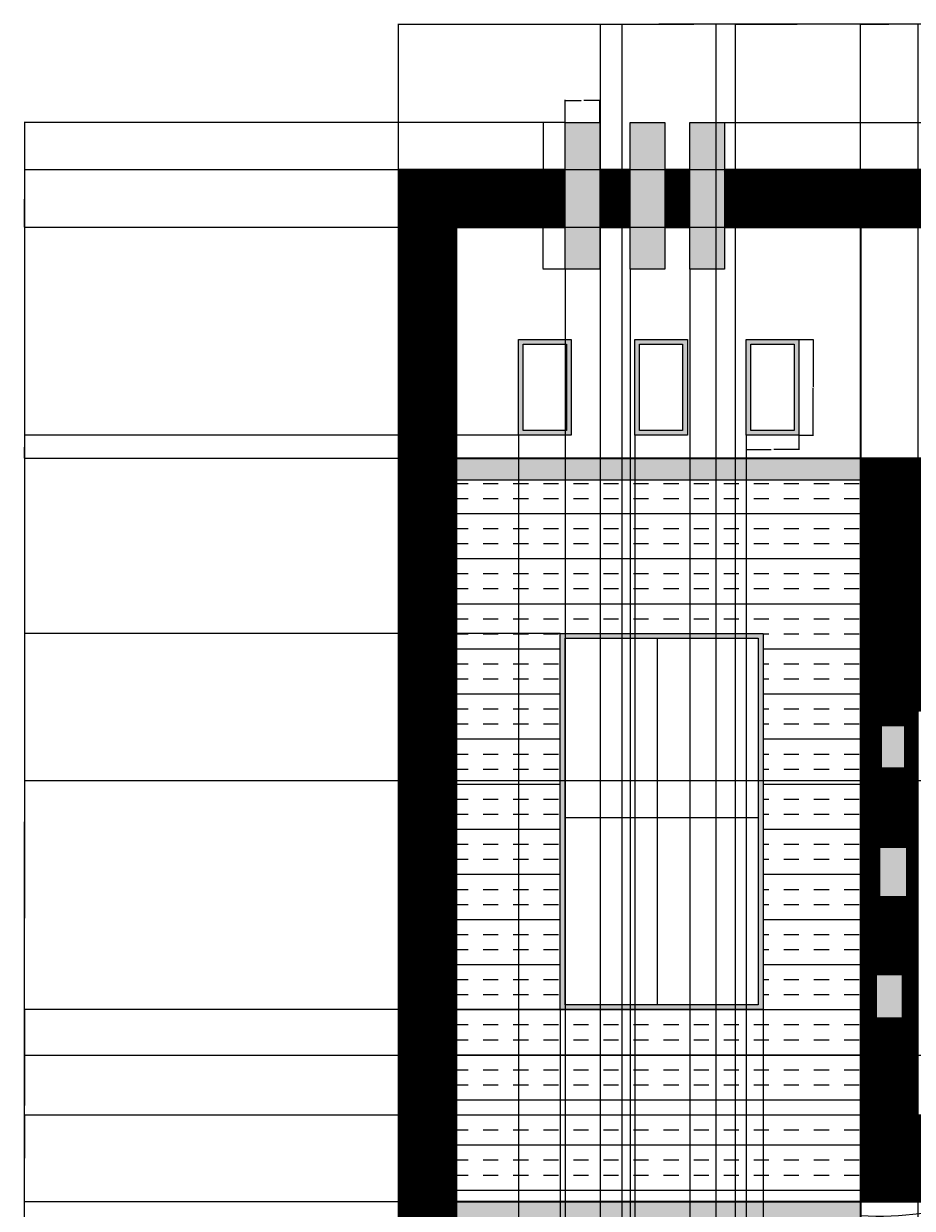
# Model space of a CAD drawing. Units: inches. Extents: x 484 to 1264, y 95 to 991.
# Tile 7 of 8: x 484 to 853, y 499 to 991. Entities that reach past the tile are written whole.
import ezdxf

# ---------------------------------------------------------------- set-up
doc = ezdxf.new("R2010")
doc.units = ezdxf.units.IN
doc.header["$MEASUREMENT"] = 0
for name, color, linetype, lineweight in [('A-ANNO-DIMS', 2, 'Continuous', 18), ('A-ELEV-TRIM', 7, 'Continuous', 18), ('A-GLAZ', 7, 'Continuous', 18), ('A-WALL', 7, 'Continuous', 35)]:
    doc.layers.add(name, color=color, linetype=linetype, lineweight=lineweight)
for name, color, linetype, lineweight, true_color in [('A-ELEV-TRIM-PATT', 40, 'Continuous', 13, 0xe7c208), ('A-WALL-CLAD-PATT', 51, 'Continuous', 13, 0xf7f281), ('A-WALL-FRAM-PATT', 158, 'Continuous', 13, 0x131d3e)]:
    doc.layers.add(name, color=color, linetype=linetype, lineweight=lineweight, true_color=true_color)
doc.styles.get("Standard").update_dxf_attribs({"font": 'arial.ttf'})
doc.dimstyles.get("Standard").update_dxf_attribs({"dimtxt": 0.18, "dimasz": 0.18, "dimexe": 0.18, "dimexo": 0.0625, "dimgap": 0.09, "dimtad": 0, "dimtih": 1, "dimtoh": 1, "dimdec": 4, "dimzin": 0, "dimdsep": 46, "dimtxsty": 'Standard', "dimcen": 0.09, "dimadec": 0, "dimazin": 0, "dimtfac": 1, "dimtdec": 4, "dimtofl": 0, "dimtmove": 0, "dimatfit": 3, "dimfxl": 1, "dimtolj": 1, "dimtzin": 0, "dimarcsym": 0})

# ---------------------------------------------------------------- blocks, each defined once
blk = doc.blocks.new('WIN-UPPER-SINGLE-LIGHT')
for points in [[(0, 39.82), (21.92, 39.82), (21.92, 0), (0, 0)], [(2, 37.82), (19.92, 37.82), (19.92, 2), (2, 2)]]:
    blk.add_lwpolyline(points, close=True)
blk = doc.blocks.new('PARAPET-ACCENT-FIN')
blk.add_lwpolyline([(0, 60.96), (14.39, 60.96), (14.39, 0), (0, 0)], close=True)
blk = doc.blocks.new('*D10')
at = {"layer": 'A-ANNO-DIMS', "color": 0, "lineweight": -2, "transparency": 16777216}
for p, q in [((806.28, 859.87), (812.37, 859.87)), ((812.19, 859.69), (812.19, 840.15)), ((812.19, 820.24), (812.19, 839.78)), ((806.28, 820.06), (812.37, 820.06))]:
    blk.add_line(p, q, dxfattribs=at)
at = {"layer": 'A-ANNO-DIMS', "color": 0, "transparency": 16777216}
for points in [[(812.16, 859.69), (812.22, 859.69), (812.19, 859.87)], [(812.16, 820.24), (812.22, 820.24), (812.19, 820.06)]]:
    blk.add_solid(points, dxfattribs=at)
at = {"layer": 'Defpoints', "color": 0, "transparency": 16777216}
for p in [(806.22, 859.87), (812.19, 859.87), (806.22, 820.06)]:
    blk.add_point(p, dxfattribs=at)
at = {"layer": 'A-ANNO-DIMS', "color": 0, "transparency": 16777216, "insert": (812.19, 839.96), "char_height": 0.18, "attachment_point": 5}
blk.add_mtext('\\A1;LIGHT 40 TYP.', dxfattribs=at)
blk = doc.blocks.new('*D11')
at = {"layer": 'A-ANNO-DIMS', "color": 0, "lineweight": -2, "transparency": 16777216}
for p, q in [((784.3, 819.99), (784.3, 813.9)), ((806.22, 819.99), (806.22, 813.9)), ((784.48, 814.08), (794.73, 814.08)), ((806.04, 814.08), (795.79, 814.08))]:
    blk.add_line(p, q, dxfattribs=at)
at = {"layer": 'A-ANNO-DIMS', "color": 0, "transparency": 16777216}
for points in [[(784.48, 814.11), (784.48, 814.05), (784.3, 814.08)], [(806.04, 814.11), (806.04, 814.05), (806.22, 814.08)]]:
    blk.add_solid(points, dxfattribs=at)
at = {"layer": 'Defpoints', "color": 0, "transparency": 16777216}
for p in [(784.3, 820.06), (806.22, 820.06), (806.22, 814.08)]:
    blk.add_point(p, dxfattribs=at)
at = {"layer": 'A-ANNO-DIMS', "color": 0, "transparency": 16777216, "insert": (795.26, 814.08), "char_height": 0.18, "attachment_point": 5}
blk.add_mtext('\\A1;22 TYP.', dxfattribs=at)
blk = doc.blocks.new('*D12')
at = {"layer": 'A-ANNO-DIMS', "color": 0, "lineweight": -2, "transparency": 16777216}
for p, q in [((709.01, 950.08), (699.74, 950.08)), ((699.92, 949.9), (699.92, 919.78)), ((699.92, 889.3), (699.92, 919.42)), ((709.01, 889.12), (699.74, 889.12))]:
    blk.add_line(p, q, dxfattribs=at)
at = {"layer": 'A-ANNO-DIMS', "color": 0, "transparency": 16777216}
for points in [[(699.89, 949.9), (699.95, 949.9), (699.92, 950.08)], [(699.89, 889.3), (699.95, 889.3), (699.92, 889.12)]]:
    blk.add_solid(points, dxfattribs=at)
at = {"layer": 'Defpoints', "color": 0, "transparency": 16777216}
for p in [(699.92, 950.08), (709.07, 950.08), (709.07, 889.12)]:
    blk.add_point(p, dxfattribs=at)
at = {"layer": 'A-ANNO-DIMS', "color": 0, "transparency": 16777216, "insert": (699.92, 919.6), "char_height": 0.18, "attachment_point": 5}
blk.add_mtext('\\A1;FIN 61 TYP.', dxfattribs=at)
blk = doc.blocks.new('*D13')
at = {"layer": 'A-ANNO-DIMS', "color": 0, "lineweight": -2, "transparency": 16777216}
for p, q in [((709.07, 950.14), (709.07, 959.4)), ((709.25, 959.22), (715.74, 959.22)), ((723.28, 959.22), (716.78, 959.22)), ((723.46, 950.14), (723.46, 959.4))]:
    blk.add_line(p, q, dxfattribs=at)
at = {"layer": 'A-ANNO-DIMS', "color": 0, "transparency": 16777216}
for points in [[(709.25, 959.25), (709.25, 959.19), (709.07, 959.22)], [(723.28, 959.25), (723.28, 959.19), (723.46, 959.22)]]:
    blk.add_solid(points, dxfattribs=at)
at = {"layer": 'Defpoints', "color": 0, "transparency": 16777216}
for p in [(723.46, 959.22), (709.07, 950.08), (723.46, 950.08)]:
    blk.add_point(p, dxfattribs=at)
at = {"layer": 'A-ANNO-DIMS', "color": 0, "transparency": 16777216, "insert": (716.26, 959.22), "char_height": 0.18, "attachment_point": 5}
blk.add_mtext('\\A1;14 TYP.', dxfattribs=at)
blk = doc.blocks.new('*D17')
at = {"layer": 'A-ANNO-DIMS', "color": 0, "lineweight": -2, "transparency": 16777216}
for p, q in [((709.01, 950.08), (484.15, 950.08)), ((484.33, 949.9), (484.33, 628.41)), ((484.33, 306.56), (484.33, 628.05)), ((595.26, 306.38), (484.15, 306.38))]:
    blk.add_line(p, q, dxfattribs=at)
at = {"layer": 'A-ANNO-DIMS', "color": 0, "transparency": 16777216}
for points in [[(484.3, 949.9), (484.36, 949.9), (484.33, 950.08)], [(484.3, 306.56), (484.36, 306.56), (484.33, 306.38)]]:
    blk.add_solid(points, dxfattribs=at)
at = {"layer": 'Defpoints', "color": 0, "transparency": 16777216}
for p in [(484.33, 950.08), (709.07, 950.08), (595.32, 306.38)]:
    blk.add_point(p, dxfattribs=at)
at = {"layer": 'A-ANNO-DIMS', "color": 0, "transparency": 16777216, "insert": (484.33, 628.23), "char_height": 0.18, "attachment_point": 5}
blk.add_mtext('\\A1;643.7', dxfattribs=at)
blk = doc.blocks.new('*D18')
at = {"layer": 'A-ANNO-DIMS', "color": 0, "lineweight": -2, "transparency": 16777216}
for p, q in [((999.88, 501.38), (1264.08, 501.38)), ((1263.9, 501.2), (1263.9, 404.07)), ((1263.9, 306.56), (1263.9, 403.7)), ((595.38, 306.38), (1264.08, 306.38))]:
    blk.add_line(p, q, dxfattribs=at)
at = {"layer": 'A-ANNO-DIMS', "color": 0, "transparency": 16777216}
for points in [[(1263.87, 501.2), (1263.93, 501.2), (1263.9, 501.38)], [(1263.87, 306.56), (1263.93, 306.56), (1263.9, 306.38)]]:
    blk.add_solid(points, dxfattribs=at)
at = {"layer": 'Defpoints', "color": 0, "transparency": 16777216}
for p in [(999.81, 501.38), (1263.9, 501.38), (595.32, 306.38)]:
    blk.add_point(p, dxfattribs=at)
at = {"layer": 'A-ANNO-DIMS', "color": 0, "transparency": 16777216, "insert": (1263.9, 403.88), "char_height": 0.18, "attachment_point": 5}
blk.add_mtext('\\A1;195', dxfattribs=at)
blk = doc.blocks.new('*D22')
at = {"layer": 'A-ANNO-DIMS', "color": 0, "lineweight": -2, "transparency": 16777216}
for p, q in [((639.81, 930.45), (639.81, 991.11)), ((639.99, 990.93), (762.52, 990.93)), ((885.63, 990.93), (763.11, 990.93)), ((885.81, 930.45), (885.81, 991.11))]:
    blk.add_line(p, q, dxfattribs=at)
at = {"layer": 'A-ANNO-DIMS', "color": 0, "transparency": 16777216}
for points in [[(639.99, 990.96), (639.99, 990.9), (639.81, 990.93)], [(885.63, 990.96), (885.63, 990.9), (885.81, 990.93)]]:
    blk.add_solid(points, dxfattribs=at)
at = {"layer": 'Defpoints', "color": 0, "transparency": 16777216}
for p in [(885.81, 990.93), (639.81, 930.38), (885.81, 930.38)]:
    blk.add_point(p, dxfattribs=at)
at = {"layer": 'A-ANNO-DIMS', "color": 0, "transparency": 16777216, "insert": (762.81, 990.93), "char_height": 0.18, "attachment_point": 5}
blk.add_mtext('\\A1;246', dxfattribs=at)
blk = doc.blocks.new('*D23')
at = {"layer": 'A-ANNO-DIMS', "color": 0, "lineweight": -2, "transparency": 16777216}
for p, q in [((663.81, 906.32), (663.81, 94.79)), ((709.07, 889.06), (709.07, 94.79)), ((663.99, 94.97), (686.04, 94.97)), ((708.89, 94.97), (686.84, 94.97))]:
    blk.add_line(p, q, dxfattribs=at)
at = {"layer": 'A-ANNO-DIMS', "color": 0, "transparency": 16777216}
for points in [[(663.99, 95), (663.99, 94.94), (663.81, 94.97)], [(708.89, 95), (708.89, 94.94), (709.07, 94.97)]]:
    blk.add_solid(points, dxfattribs=at)
at = {"layer": 'Defpoints', "color": 0, "transparency": 16777216}
for p in [(663.81, 906.38), (709.07, 889.12), (709.07, 94.97)]:
    blk.add_point(p, dxfattribs=at)
at = {"layer": 'A-ANNO-DIMS', "color": 0, "transparency": 16777216, "insert": (686.44, 94.97), "char_height": 0.18, "attachment_point": 5}
blk.add_mtext('\\A1;45.25', dxfattribs=at)
blk = doc.blocks.new('*D24')
at = {"layer": 'A-ANNO-DIMS', "color": 0, "lineweight": -2, "transparency": 16777216}
for p, q in [((709.07, 889.06), (709.07, 94.79)), ((736.12, 889.06), (736.12, 94.79)), ((709.25, 94.97), (722.2, 94.97)), ((735.94, 94.97), (722.99, 94.97))]:
    blk.add_line(p, q, dxfattribs=at)
at = {"layer": 'A-ANNO-DIMS', "color": 0, "transparency": 16777216}
for points in [[(709.25, 95), (709.25, 94.94), (709.07, 94.97)], [(735.94, 95), (735.94, 94.94), (736.12, 94.97)]]:
    blk.add_solid(points, dxfattribs=at)
at = {"layer": 'Defpoints', "color": 0, "transparency": 16777216}
for p in [(709.07, 889.12), (736.12, 889.12), (736.12, 94.97)]:
    blk.add_point(p, dxfattribs=at)
at = {"layer": 'A-ANNO-DIMS', "color": 0, "transparency": 16777216, "insert": (722.59, 94.97), "char_height": 0.18, "attachment_point": 5}
blk.add_mtext('\\A1;27.05', dxfattribs=at)
blk = doc.blocks.new('*D25')
at = {"layer": 'A-ANNO-DIMS', "color": 0, "lineweight": -2, "transparency": 16777216}
for p, q in [((736.12, 889.06), (736.12, 94.79)), ((760.87, 889.06), (760.87, 94.79)), ((736.3, 94.97), (748.1, 94.97)), ((760.69, 94.97), (748.89, 94.97))]:
    blk.add_line(p, q, dxfattribs=at)
at = {"layer": 'A-ANNO-DIMS', "color": 0, "transparency": 16777216}
for points in [[(736.3, 95), (736.3, 94.94), (736.12, 94.97)], [(760.69, 95), (760.69, 94.94), (760.87, 94.97)]]:
    blk.add_solid(points, dxfattribs=at)
at = {"layer": 'Defpoints', "color": 0, "transparency": 16777216}
for p in [(736.12, 889.12), (760.87, 889.12), (760.87, 94.97)]:
    blk.add_point(p, dxfattribs=at)
at = {"layer": 'A-ANNO-DIMS', "color": 0, "transparency": 16777216, "insert": (748.49, 94.97), "char_height": 0.18, "attachment_point": 5}
blk.add_mtext('\\A1;24.75', dxfattribs=at)
blk = doc.blocks.new('*D26')
at = {"layer": 'A-ANNO-DIMS', "color": 0, "lineweight": -2, "transparency": 16777216}
for p, q in [((689.66, 819.99), (689.66, 94.79)), ((663.81, 810.32), (663.81, 94.79)), ((663.99, 94.97), (676.27, 94.97)), ((689.48, 94.97), (677.2, 94.97))]:
    blk.add_line(p, q, dxfattribs=at)
at = {"layer": 'A-ANNO-DIMS', "color": 0, "transparency": 16777216}
for points in [[(663.99, 95), (663.99, 94.94), (663.81, 94.97)], [(689.48, 95), (689.48, 94.94), (689.66, 94.97)]]:
    blk.add_solid(points, dxfattribs=at)
at = {"layer": 'Defpoints', "color": 0, "transparency": 16777216}
for p in [(689.66, 820.06), (663.81, 810.38), (689.66, 94.97)]:
    blk.add_point(p, dxfattribs=at)
at = {"layer": 'A-ANNO-DIMS', "color": 0, "transparency": 16777216, "insert": (676.74, 94.97), "char_height": 0.18, "attachment_point": 5}
blk.add_mtext('\\A1;25.846', dxfattribs=at)
blk = doc.blocks.new('*D27')
at = {"layer": 'A-ANNO-DIMS', "color": 0, "lineweight": -2, "transparency": 16777216}
for p, q in [((689.66, 819.99), (689.66, 94.79)), ((737.98, 819.99), (737.98, 94.79)), ((689.84, 94.97), (713.42, 94.97)), ((737.8, 94.97), (714.22, 94.97))]:
    blk.add_line(p, q, dxfattribs=at)
at = {"layer": 'A-ANNO-DIMS', "color": 0, "transparency": 16777216}
for points in [[(689.84, 95), (689.84, 94.94), (689.66, 94.97)], [(737.8, 95), (737.8, 94.94), (737.98, 94.97)]]:
    blk.add_solid(points, dxfattribs=at)
at = {"layer": 'Defpoints', "color": 0, "transparency": 16777216}
for p in [(689.66, 820.06), (737.98, 820.06), (737.98, 94.97)]:
    blk.add_point(p, dxfattribs=at)
at = {"layer": 'A-ANNO-DIMS', "color": 0, "transparency": 16777216, "insert": (713.82, 94.97), "char_height": 0.18, "attachment_point": 5}
blk.add_mtext('\\A1;48.32', dxfattribs=at)
blk = doc.blocks.new('*D28')
at = {"layer": 'A-ANNO-DIMS', "color": 0, "lineweight": -2, "transparency": 16777216}
for p, q in [((737.98, 819.99), (737.98, 94.79)), ((784.3, 819.99), (784.3, 94.79)), ((738.16, 94.97), (760.67, 94.97)), ((784.12, 94.97), (761.61, 94.97))]:
    blk.add_line(p, q, dxfattribs=at)
at = {"layer": 'A-ANNO-DIMS', "color": 0, "transparency": 16777216}
for points in [[(738.16, 95), (738.16, 94.94), (737.98, 94.97)], [(784.12, 95), (784.12, 94.94), (784.3, 94.97)]]:
    blk.add_solid(points, dxfattribs=at)
at = {"layer": 'Defpoints', "color": 0, "transparency": 16777216}
for p in [(737.98, 820.06), (784.3, 820.06), (784.3, 94.97)]:
    blk.add_point(p, dxfattribs=at)
at = {"layer": 'A-ANNO-DIMS', "color": 0, "transparency": 16777216, "insert": (761.14, 94.97), "char_height": 0.18, "attachment_point": 5}
blk.add_mtext('\\A1;46.325', dxfattribs=at)
blk = doc.blocks.new('*D29')
at = {"layer": 'A-ANNO-DIMS', "color": 0, "lineweight": -2, "transparency": 16777216}
for p, q in [((831.81, 906.32), (831.81, 94.79)), ((784.3, 819.99), (784.3, 94.79)), ((784.48, 94.97), (807.68, 94.97)), ((831.63, 94.97), (808.44, 94.97))]:
    blk.add_line(p, q, dxfattribs=at)
at = {"layer": 'A-ANNO-DIMS', "color": 0, "transparency": 16777216}
for points in [[(784.48, 95), (784.48, 94.94), (784.3, 94.97)], [(831.63, 95), (831.63, 94.94), (831.81, 94.97)]]:
    blk.add_solid(points, dxfattribs=at)
at = {"layer": 'Defpoints', "color": 0, "transparency": 16777216}
for p in [(831.81, 906.38), (784.3, 820.06), (831.81, 94.97)]:
    blk.add_point(p, dxfattribs=at)
at = {"layer": 'A-ANNO-DIMS', "color": 0, "transparency": 16777216, "insert": (808.06, 94.97), "char_height": 0.18, "attachment_point": 5}
blk.add_mtext('\\A1;47.51', dxfattribs=at)
blk = doc.blocks.new('*D30')
at = {"layer": 'A-ANNO-DIMS', "color": 0, "lineweight": -2, "transparency": 16777216}
for p, q in [((689.6, 820.06), (484.15, 820.06)), ((484.33, 819.88), (484.33, 815.4)), ((484.33, 810.56), (484.33, 815.04)), ((663.75, 810.38), (484.15, 810.38))]:
    blk.add_line(p, q, dxfattribs=at)
at = {"layer": 'A-ANNO-DIMS', "color": 0, "transparency": 16777216}
for points in [[(484.3, 819.88), (484.36, 819.88), (484.33, 820.06)], [(484.3, 810.56), (484.36, 810.56), (484.33, 810.38)]]:
    blk.add_solid(points, dxfattribs=at)
at = {"layer": 'Defpoints', "color": 0, "transparency": 16777216}
for p in [(484.33, 820.06), (689.66, 820.06), (663.81, 810.38)]:
    blk.add_point(p, dxfattribs=at)
at = {"layer": 'A-ANNO-DIMS', "color": 0, "transparency": 16777216, "insert": (484.33, 815.22), "char_height": 0.18, "attachment_point": 5}
blk.add_mtext('\\A1;9.672', dxfattribs=at)
blk = doc.blocks.new('*D31')
at = {"layer": 'A-ANNO-DIMS', "color": 0, "lineweight": -2, "transparency": 16777216}
for p, q in [((760.93, 950.08), (1264.08, 950.08)), ((1263.9, 949.9), (1263.9, 940.41)), ((1263.9, 930.56), (1263.9, 940.05)), ((885.88, 930.38), (1264.08, 930.38))]:
    blk.add_line(p, q, dxfattribs=at)
at = {"layer": 'A-ANNO-DIMS', "color": 0, "transparency": 16777216}
for points in [[(1263.87, 949.9), (1263.93, 949.9), (1263.9, 950.08)], [(1263.87, 930.56), (1263.93, 930.56), (1263.9, 930.38)]]:
    blk.add_solid(points, dxfattribs=at)
at = {"layer": 'Defpoints', "color": 0, "transparency": 16777216}
for p in [(760.87, 950.08), (1263.9, 950.08), (885.81, 930.38)]:
    blk.add_point(p, dxfattribs=at)
at = {"layer": 'A-ANNO-DIMS', "color": 0, "transparency": 16777216, "insert": (1263.9, 940.23), "char_height": 0.18, "attachment_point": 5}
blk.add_mtext('\\A1;19.694', dxfattribs=at)
blk = doc.blocks.new('*D32')
at = {"layer": 'A-ANNO-DIMS', "color": 0, "lineweight": -2, "transparency": 16777216}
for p, q in [((885.75, 930.38), (484.15, 930.38)), ((484.33, 930.2), (484.33, 918.56)), ((484.33, 906.56), (484.33, 918.2)), ((885.75, 906.38), (484.15, 906.38))]:
    blk.add_line(p, q, dxfattribs=at)
at = {"layer": 'A-ANNO-DIMS', "color": 0, "transparency": 16777216}
for points in [[(484.3, 930.2), (484.36, 930.2), (484.33, 930.38)], [(484.3, 906.56), (484.36, 906.56), (484.33, 906.38)]]:
    blk.add_solid(points, dxfattribs=at)
at = {"layer": 'Defpoints', "color": 0, "transparency": 16777216}
for p in [(484.33, 930.38), (885.81, 930.38), (885.81, 906.38)]:
    blk.add_point(p, dxfattribs=at)
at = {"layer": 'A-ANNO-DIMS', "color": 0, "transparency": 16777216, "insert": (484.33, 918.38), "char_height": 0.18, "attachment_point": 5}
blk.add_mtext('\\A1;24', dxfattribs=at)
blk = doc.blocks.new('*D33')
at = {"layer": 'A-ANNO-DIMS', "color": 0, "lineweight": -2, "transparency": 16777216}
for p, q in [((639.81, 930.32), (639.81, 94.79)), ((663.81, 810.32), (663.81, 94.79)), ((639.99, 94.97), (651.59, 94.97)), ((663.63, 94.97), (652.03, 94.97))]:
    blk.add_line(p, q, dxfattribs=at)
at = {"layer": 'A-ANNO-DIMS', "color": 0, "transparency": 16777216}
for points in [[(639.99, 95), (639.99, 94.94), (639.81, 94.97)], [(663.63, 95), (663.63, 94.94), (663.81, 94.97)]]:
    blk.add_solid(points, dxfattribs=at)
at = {"layer": 'Defpoints', "color": 0, "transparency": 16777216}
for p in [(639.81, 930.38), (663.81, 810.38), (663.81, 94.97)]:
    blk.add_point(p, dxfattribs=at)
at = {"layer": 'A-ANNO-DIMS', "color": 0, "transparency": 16777216, "insert": (651.81, 94.97), "char_height": 0.18, "attachment_point": 5}
blk.add_mtext('\\A1;24', dxfattribs=at)
blk = doc.blocks.new('*D34')
at = {"layer": 'A-ANNO-DIMS', "color": 0, "lineweight": -2, "transparency": 16777216}
for p, q in [((706.98, 581.28), (484.15, 581.28)), ((484.33, 581.1), (484.33, 541.51)), ((484.33, 501.56), (484.33, 541.15)), ((663.75, 501.38), (484.15, 501.38))]:
    blk.add_line(p, q, dxfattribs=at)
at = {"layer": 'A-ANNO-DIMS', "color": 0, "transparency": 16777216}
for points in [[(484.3, 581.1), (484.36, 581.1), (484.33, 581.28)], [(484.3, 501.56), (484.36, 501.56), (484.33, 501.38)]]:
    blk.add_solid(points, dxfattribs=at)
at = {"layer": 'Defpoints', "color": 0, "transparency": 16777216}
for p in [(484.33, 581.28), (707.04, 581.28), (663.81, 501.38)]:
    blk.add_point(p, dxfattribs=at)
at = {"layer": 'A-ANNO-DIMS', "color": 0, "transparency": 16777216, "insert": (484.33, 541.33), "char_height": 0.18, "attachment_point": 5}
blk.add_mtext('\\A1;79.89', dxfattribs=at)
blk = doc.blocks.new('*D35')
at = {"layer": 'A-ANNO-DIMS', "color": 0, "lineweight": -2, "transparency": 16777216}
for p, q in [((706.98, 737.65), (484.15, 737.65)), ((484.33, 737.47), (484.33, 659.65)), ((484.33, 581.46), (484.33, 659.28)), ((706.98, 581.28), (484.15, 581.28))]:
    blk.add_line(p, q, dxfattribs=at)
at = {"layer": 'A-ANNO-DIMS', "color": 0, "transparency": 16777216}
for points in [[(484.3, 737.47), (484.36, 737.47), (484.33, 737.65)], [(484.3, 581.46), (484.36, 581.46), (484.33, 581.28)]]:
    blk.add_solid(points, dxfattribs=at)
at = {"layer": 'Defpoints', "color": 0, "transparency": 16777216}
for p in [(484.33, 737.65), (707.04, 737.65), (707.04, 581.28)]:
    blk.add_point(p, dxfattribs=at)
at = {"layer": 'A-ANNO-DIMS', "color": 0, "transparency": 16777216, "insert": (484.33, 659.46), "char_height": 0.18, "attachment_point": 5}
blk.add_mtext('\\A1;156.37', dxfattribs=at)
blk = doc.blocks.new('*D36')
at = {"layer": 'A-ANNO-DIMS', "color": 0, "lineweight": -2, "transparency": 16777216}
for p, q in [((707.04, 581.21), (707.04, 94.79)), ((663.81, 501.32), (663.81, 94.79)), ((663.99, 94.97), (685.03, 94.97)), ((706.86, 94.97), (685.82, 94.97))]:
    blk.add_line(p, q, dxfattribs=at)
at = {"layer": 'A-ANNO-DIMS', "color": 0, "transparency": 16777216}
for points in [[(663.99, 95), (663.99, 94.94), (663.81, 94.97)], [(706.86, 95), (706.86, 94.94), (707.04, 94.97)]]:
    blk.add_solid(points, dxfattribs=at)
at = {"layer": 'Defpoints', "color": 0, "transparency": 16777216}
for p in [(707.04, 581.28), (663.81, 501.38), (707.04, 94.97)]:
    blk.add_point(p, dxfattribs=at)
at = {"layer": 'A-ANNO-DIMS', "color": 0, "transparency": 16777216, "insert": (685.43, 94.97), "char_height": 0.18, "attachment_point": 5}
blk.add_mtext('\\A1;43.22', dxfattribs=at)
blk = doc.blocks.new('*D37')
at = {"layer": 'A-ANNO-DIMS', "color": 0, "lineweight": -2, "transparency": 16777216}
for p, q in [((707.04, 581.21), (707.04, 94.79)), ((791.36, 581.21), (791.36, 94.79)), ((707.22, 94.97), (748.81, 94.97)), ((791.18, 94.97), (749.59, 94.97))]:
    blk.add_line(p, q, dxfattribs=at)
at = {"layer": 'A-ANNO-DIMS', "color": 0, "transparency": 16777216}
for points in [[(707.22, 95), (707.22, 94.94), (707.04, 94.97)], [(791.18, 95), (791.18, 94.94), (791.36, 94.97)]]:
    blk.add_solid(points, dxfattribs=at)
at = {"layer": 'Defpoints', "color": 0, "transparency": 16777216}
for p in [(707.04, 581.28), (791.36, 581.28), (791.36, 94.97)]:
    blk.add_point(p, dxfattribs=at)
at = {"layer": 'A-ANNO-DIMS', "color": 0, "transparency": 16777216, "insert": (749.2, 94.97), "char_height": 0.18, "attachment_point": 5}
blk.add_mtext('\\A1;84.32', dxfattribs=at)
blk = doc.blocks.new('*D38')
at = {"layer": 'A-ANNO-DIMS', "color": 0, "lineweight": -2, "transparency": 16777216}
for p, q in [((899.62, 676.35), (484.15, 676.35)), ((484.33, 676.17), (484.33, 619.48)), ((484.33, 562.44), (484.33, 619.12)), ((899.62, 562.26), (484.15, 562.26))]:
    blk.add_line(p, q, dxfattribs=at)
at = {"layer": 'A-ANNO-DIMS', "color": 0, "transparency": 16777216}
for points in [[(484.3, 676.17), (484.36, 676.17), (484.33, 676.35)], [(484.3, 562.44), (484.36, 562.44), (484.33, 562.26)]]:
    blk.add_solid(points, dxfattribs=at)
at = {"layer": 'Defpoints', "color": 0, "transparency": 16777216}
for p in [(484.33, 676.35), (899.68, 676.35), (899.68, 562.26)]:
    blk.add_point(p, dxfattribs=at)
at = {"layer": 'A-ANNO-DIMS', "color": 0, "transparency": 16777216, "insert": (484.33, 619.3), "char_height": 0.18, "attachment_point": 5}
blk.add_mtext('\\A1;114.1', dxfattribs=at)
blk = doc.blocks.new('*D39')
at = {"layer": 'A-ANNO-DIMS', "color": 0, "lineweight": -2, "transparency": 16777216}
for p, q in [((899.62, 562.26), (484.15, 562.26)), ((484.33, 562.08), (484.33, 550)), ((484.33, 537.56), (484.33, 549.64)), ((855.75, 537.38), (484.15, 537.38))]:
    blk.add_line(p, q, dxfattribs=at)
at = {"layer": 'A-ANNO-DIMS', "color": 0, "transparency": 16777216}
for points in [[(484.3, 562.08), (484.36, 562.08), (484.33, 562.26)], [(484.3, 537.56), (484.36, 537.56), (484.33, 537.38)]]:
    blk.add_solid(points, dxfattribs=at)
at = {"layer": 'Defpoints', "color": 0, "transparency": 16777216}
for p in [(484.33, 562.26), (899.68, 562.26), (855.81, 537.38)]:
    blk.add_point(p, dxfattribs=at)
at = {"layer": 'A-ANNO-DIMS', "color": 0, "transparency": 16777216, "insert": (484.33, 549.82), "char_height": 0.18, "attachment_point": 5}
blk.add_mtext('\\A1;24.87', dxfattribs=at)
blk = doc.blocks.new('*D44')
at = {"layer": 'A-ANNO-DIMS', "color": 0, "lineweight": -2, "transparency": 16777216}
for p, q in [((999.75, 537.38), (484.15, 537.38)), ((484.33, 537.2), (484.33, 519.57)), ((484.33, 501.56), (484.33, 519.2)), ((999.75, 501.38), (484.15, 501.38))]:
    blk.add_line(p, q, dxfattribs=at)
at = {"layer": 'A-ANNO-DIMS', "color": 0, "transparency": 16777216}
for points in [[(484.3, 537.2), (484.36, 537.2), (484.33, 537.38)], [(484.3, 501.56), (484.36, 501.56), (484.33, 501.38)]]:
    blk.add_solid(points, dxfattribs=at)
at = {"layer": 'Defpoints', "color": 0, "transparency": 16777216}
for p in [(484.33, 537.38), (999.81, 537.38), (999.81, 501.38)]:
    blk.add_point(p, dxfattribs=at)
at = {"layer": 'A-ANNO-DIMS', "color": 0, "transparency": 16777216, "insert": (484.33, 519.38), "char_height": 0.18, "attachment_point": 5}
blk.add_mtext('\\A1;36', dxfattribs=at)
blk = doc.blocks.new('*D45')
at = {"layer": 'A-ANNO-DIMS', "color": 0, "lineweight": -2, "transparency": 16777216}
for p, q in [((732.77, 470.83), (732.77, 991.11)), ((732.95, 990.93), (755.94, 990.93)), ((779.73, 990.93), (756.74, 990.93)), ((779.91, 470.83), (779.91, 991.11))]:
    blk.add_line(p, q, dxfattribs=at)
at = {"layer": 'A-ANNO-DIMS', "color": 0, "transparency": 16777216}
for points in [[(732.95, 990.96), (732.95, 990.9), (732.77, 990.93)], [(779.73, 990.96), (779.73, 990.9), (779.91, 990.93)]]:
    blk.add_solid(points, dxfattribs=at)
at = {"layer": 'Defpoints', "color": 0, "transparency": 16777216}
for p in [(779.91, 990.93), (732.77, 470.76), (779.91, 470.76)]:
    blk.add_point(p, dxfattribs=at)
at = {"layer": 'A-ANNO-DIMS', "color": 0, "transparency": 16777216, "insert": (756.34, 990.93), "char_height": 0.18, "attachment_point": 5}
blk.add_mtext('\\A1;47.13', dxfattribs=at)
blk = doc.blocks.new('*D46')
at = {"layer": 'A-ANNO-DIMS', "color": 0, "lineweight": -2, "transparency": 16777216}
for p, q in [((779.91, 470.83), (779.91, 991.11)), ((780.09, 990.93), (805.48, 990.93)), ((831.63, 990.93), (806.24, 990.93)), ((831.81, 492.45), (831.81, 991.11))]:
    blk.add_line(p, q, dxfattribs=at)
at = {"layer": 'A-ANNO-DIMS', "color": 0, "transparency": 16777216}
for points in [[(780.09, 990.96), (780.09, 990.9), (779.91, 990.93)], [(831.63, 990.96), (831.63, 990.9), (831.81, 990.93)]]:
    blk.add_solid(points, dxfattribs=at)
at = {"layer": 'Defpoints', "color": 0, "transparency": 16777216}
for p in [(831.81, 990.93), (831.81, 492.38), (779.91, 470.76)]:
    blk.add_point(p, dxfattribs=at)
at = {"layer": 'A-ANNO-DIMS', "color": 0, "transparency": 16777216, "insert": (805.86, 990.93), "char_height": 0.18, "attachment_point": 5}
blk.add_mtext('\\A1;51.91', dxfattribs=at)
blk = doc.blocks.new('*D52')
at = {"layer": 'A-ANNO-DIMS', "color": 0, "lineweight": -2, "transparency": 16777216}
for p, q in [((723.81, 420.45), (723.81, 991.11)), ((723.99, 990.93), (747.59, 990.93)), ((771.63, 990.93), (748.04, 990.93)), ((771.81, 420.45), (771.81, 991.11))]:
    blk.add_line(p, q, dxfattribs=at)
at = {"layer": 'A-ANNO-DIMS', "color": 0, "transparency": 16777216}
for points in [[(723.99, 990.96), (723.99, 990.9), (723.81, 990.93)], [(771.63, 990.96), (771.63, 990.9), (771.81, 990.93)]]:
    blk.add_solid(points, dxfattribs=at)
at = {"layer": 'Defpoints', "color": 0, "transparency": 16777216}
for p in [(771.81, 990.93), (723.81, 420.38), (771.81, 420.38)]:
    blk.add_point(p, dxfattribs=at)
at = {"layer": 'A-ANNO-DIMS', "color": 0, "transparency": 16777216, "insert": (747.81, 990.93), "char_height": 0.18, "attachment_point": 5}
blk.add_mtext('\\A1;48', dxfattribs=at)
blk = doc.blocks.new('*D54')
at = {"layer": 'A-ANNO-DIMS', "color": 0, "lineweight": -2, "transparency": 16777216}
for p, q in [((831.81, 420.5), (831.81, 991.11)), ((831.99, 990.93), (843.59, 990.93)), ((855.63, 990.93), (844.03, 990.93)), ((855.81, 420.5), (855.81, 991.11))]:
    blk.add_line(p, q, dxfattribs=at)
at = {"layer": 'A-ANNO-DIMS', "color": 0, "transparency": 16777216}
for points in [[(831.99, 990.96), (831.99, 990.9), (831.81, 990.93)], [(855.63, 990.96), (855.63, 990.9), (855.81, 990.93)]]:
    blk.add_solid(points, dxfattribs=at)
at = {"layer": 'Defpoints', "color": 0, "transparency": 16777216}
for p in [(855.81, 990.93), (831.81, 420.44), (855.81, 420.44)]:
    blk.add_point(p, dxfattribs=at)
at = {"layer": 'A-ANNO-DIMS', "color": 0, "transparency": 16777216, "insert": (843.81, 990.93), "char_height": 0.18, "attachment_point": 5}
blk.add_mtext('\\A1;24', dxfattribs=at)

msp = doc.modelspace()

# ---------------------------------------------------------------- hatches: boundary and pattern name
at = {"layer": 'A-ELEV-TRIM-PATT'}
h = msp.add_hatch(color=256, dxfattribs=at)
h.dxf.hatch_style = 1
h.paths.add_polyline_path([(791.3605, 737.6508), (707.038, 737.6508), (707.038, 581.2764), (791.3605, 581.2764)])
h.paths.add_polyline_path([(789.3605, 735.6508), (789.3605, 583.2764), (709.038, 583.2764), (709.038, 735.6508)], flags=16)
h.paths.add_polyline_path([(850.1752, 699.3334), (840.6401, 699.3334), (840.6401, 681.6082), (850.1752, 681.6082)])
h.paths.add_polyline_path([(850.9809, 648.8447), (839.9453, 648.8447), (839.9453, 628.2143), (850.9809, 628.2143)])
h.paths.add_polyline_path([(849.208, 595.8059), (838.5284, 595.8059), (838.5284, 577.6654), (849.208, 577.6654)])
h.paths.add_polyline_path([(723.4575, 950.079), (709.0683, 950.079), (709.0683, 889.1187), (723.4575, 889.1187)])
h.paths.add_polyline_path([(750.5092, 950.079), (736.12, 950.079), (736.12, 889.1187), (750.5092, 889.1187)])
h.paths.add_polyline_path([(775.2587, 950.079), (760.8695, 950.079), (760.8695, 889.1187), (775.2587, 889.1187)])
h.paths.add_polyline_path([(759.8948, 859.8728), (737.9777, 859.8728), (737.9777, 820.0562), (759.8948, 820.0562)])
h.paths.add_polyline_path([(757.8948, 822.0562), (739.9777, 822.0562), (739.9777, 857.8728), (757.8948, 857.8728)], flags=16)
h.paths.add_polyline_path([(806.2195, 859.8728), (784.3024, 859.8728), (784.3024, 820.0562), (806.2195, 820.0562)])
h.paths.add_polyline_path([(786.3024, 857.8728), (804.2195, 857.8728), (804.2195, 822.0562), (786.3024, 822.0562)], flags=16)
h.paths.add_polyline_path([(711.5775, 859.8728), (689.6604, 859.8728), (689.6604, 820.0562), (711.5775, 820.0562)])
h.paths.add_polyline_path([(709.5775, 822.0562), (691.6604, 822.0562), (691.6604, 857.8728), (709.5775, 857.8728)], flags=16)
h.paths.add_polyline_path([(831.8147, 810.3846), (663.8147, 810.3846), (663.8147, 801.3846), (831.8147, 801.3846)])
h.paths.add_polyline_path([(831.8147, 501.3846), (663.8147, 501.3846), (663.8147, 492.3846), (831.8147, 492.3846)])
h.paths.add_polyline_path([(779.9074, 470.7627), (732.7744, 470.7627), (732.7744, 420.3846), (734.7744, 420.3846), (734.7744, 468.7627), (777.9074, 468.7627), (777.9074, 420.3846), (779.9074, 420.3846)])
h.paths.add_polyline_path([(779.9074, 420.3846), (777.9074, 420.3846), (777.9074, 414.1588), (771.8147, 414.1588), (771.8147, 412.1588), (779.9074, 412.1588)])
at = {"layer": 'A-WALL-CLAD-PATT'}
h = msp.add_hatch(dxfattribs=at)
h.set_pattern_fill('INSUL', color=256, scale=50)
h.paths.add_polyline_path([(831.8147, 801.3846), (663.8147, 801.3846), (663.8147, 501.3846), (831.8147, 501.3846)])
h.paths.add_polyline_path([(707.038, 737.6508), (791.3605, 737.6508), (791.3605, 581.2764), (707.038, 581.2764)], flags=16)
h.paths.add_polyline_path([(709.038, 735.6508), (789.3605, 735.6508), (789.3605, 583.2764), (709.038, 583.2764)], flags=0)
at = {"layer": 'A-WALL-FRAM-PATT'}
h = msp.add_hatch(dxfattribs=at)
h.set_pattern_fill('ANSI31', color=256)
h.paths.add_polyline_path([(999.8147, 810.3846), (831.8147, 810.3846), (831.8147, 501.3846), (999.8147, 501.3846), (999.8147, 537.3846), (855.8147, 537.3846), (855.8147, 705.3846), (999.8147, 705.3846)])
h.paths.add_polyline_path([(850.1752, 699.3334), (850.1752, 681.6082), (840.6401, 681.6082), (840.6401, 699.3334)], flags=16)
h.paths.add_polyline_path([(850.9809, 648.8447), (850.9809, 628.2143), (839.9453, 628.2143), (839.9453, 648.8447)], flags=16)
h.paths.add_polyline_path([(849.208, 595.8059), (849.208, 577.6654), (838.5284, 577.6654), (838.5284, 595.8059)], flags=16)
h.paths.add_polyline_path([(663.8147, 906.3846), (709.0683, 906.3846), (709.0683, 930.3846), (639.8147, 930.3846), (639.8147, 408.3846), (663.8147, 408.3846)])
h.paths.add_polyline_path([(885.8147, 930.3846), (775.2587, 930.3846), (775.2587, 906.3846), (885.8147, 906.3846)])
h.paths.add_polyline_path([(760.8695, 930.3846), (750.5092, 930.3846), (750.5092, 906.3846), (760.8695, 906.3846)])
h.paths.add_polyline_path([(736.12, 930.3846), (723.4575, 930.3846), (723.4575, 906.3846), (736.12, 906.3846)])

# ---------------------------------------------------------------- linework, layer by layer
at = {"layer": 'A-ELEV-TRIM'}
msp.add_line((831.8147, 801.3846), (663.8147, 801.3846), dxfattribs=at)
for points in [[(840.6401, 699.3334), (850.1752, 699.3334), (850.1752, 681.6082), (840.6401, 681.6082)], [(839.9453, 648.8447), (850.9809, 648.8447), (850.9809, 628.2143), (839.9453, 628.2143)], [(838.5284, 595.8059), (849.208, 595.8059), (849.208, 577.6654), (838.5284, 577.6654)]]:
    msp.add_lwpolyline(points, close=True, dxfattribs=at)
msp.add_ellipse((839.1596, 504.6689), major_axis=(-35.8241, 0), ratio=0.25748145, start_param=1.36430507, end_param=2.77754981, dxfattribs=at)
at = {"layer": 'A-GLAZ'}
for p, q in [((747.367, 735.6508), (747.367, 583.2764)), ((709.038, 661.062), (789.3605, 661.062))]:
    msp.add_line(p, q, dxfattribs=at)
for points in [[(707.038, 737.6508), (791.3605, 737.6508), (791.3605, 581.2764), (707.038, 581.2764)], [(709.038, 735.6508), (789.3605, 735.6508), (789.3605, 583.2764), (709.038, 583.2764)]]:
    msp.add_lwpolyline(points, close=True, dxfattribs=at)
at = {"layer": 'A-WALL'}
for p, q in [((639.8147, 930.3846), (639.8147, 408.3846)), ((709.0683, 930.3846), (639.8147, 930.3846)), ((736.12, 930.3846), (723.4575, 930.3846)), ((760.8695, 930.3846), (750.5092, 930.3846)), ((885.8147, 930.3846), (775.2587, 930.3846)), ((663.8147, 906.3846), (663.8147, 408.3846)), ((709.0683, 906.3846), (663.8147, 906.3846)), ((736.12, 906.3846), (723.4575, 906.3846)), ((760.8695, 906.3846), (750.5092, 906.3846)), ((885.8147, 906.3846), (775.2587, 906.3846)), ((831.8147, 906.3846), (831.8147, 491.1649)), ((999.8147, 810.3846), (663.8147, 810.3846)), ((999.8147, 501.3846), (663.8147, 501.3846))]:
    msp.add_line(p, q, dxfattribs=at)

# ---------------------------------------------------------------- block references
at = {"layer": 'A-ELEV-TRIM'}
for p in [(709.0683, 889.1187), (736.12, 889.1187), (760.8695, 889.1187)]:
    msp.add_blockref('PARAPET-ACCENT-FIN', p, dxfattribs=at)
at = {"layer": 'A-GLAZ'}
for p in [(689.6604, 820.0562), (737.9777, 820.0562), (784.3024, 820.0562)]:
    msp.add_blockref('WIN-UPPER-SINGLE-LIGHT', p, dxfattribs=at)

# ---------------------------------------------------------------- dimensions: what is measured, and where the dimension line sits
at = {"layer": 'A-ANNO-DIMS'}
for base, p1, p2, override, picture, middle in [((885.8147, 990.929), (639.8147, 930.3846), (885.8147, 930.3846), {"dimdec": 0, "dimlfac": 1, "dimrnd": 0, "dimzin": 0, "dimdsep": 46, "dimlunit": 2}, '*D22', (762.8147, 990.929)), ((771.8147, 990.929), (723.8147, 420.3846), (771.8147, 420.3846), {"dimdec": 0, "dimlfac": 1, "dimrnd": 0, "dimzin": 0, "dimdsep": 46, "dimlunit": 2}, '*D52', (747.8147, 990.929)), ((779.9074, 990.929), (732.7744, 470.7627), (779.9074, 470.7627), {"dimdec": 2, "dimlfac": 1, "dimrnd": 0, "dimzin": 0, "dimdsep": 46, "dimlunit": 2}, '*D45', (756.3409, 990.929)), ((831.8147, 990.929), (779.9074, 470.7627), (831.8147, 492.3846), {"dimdec": 2, "dimlfac": 1, "dimrnd": 0, "dimzin": 0, "dimdsep": 46, "dimlunit": 2}, '*D46', (805.8611, 990.929)), ((855.8147, 990.929), (831.8147, 420.4387), (855.8147, 420.4387), {"dimdec": 0, "dimlfac": 1, "dimrnd": 0, "dimzin": 0, "dimdsep": 46, "dimlunit": 2}, '*D54', (843.8147, 990.929)), ((663.8147, 94.9714), (639.8147, 930.3846), (663.8147, 810.3846), {"dimdec": 0, "dimlfac": 1, "dimrnd": 0, "dimzin": 0, "dimdsep": 46, "dimlunit": 2}, '*D33', (651.8147, 94.9714)), ((709.0683, 94.9714), (663.8147, 906.3846), (709.0683, 889.1187), {"dimdec": 2, "dimlfac": 1, "dimrnd": 0, "dimzin": 0, "dimdsep": 46, "dimlunit": 2}, '*D23', (686.4415, 94.9714)), ((831.8147, 94.9714), (784.3024, 820.0562), (831.8147, 906.3846), {"dimdec": 2, "dimlfac": 1, "dimrnd": 0, "dimzin": 0, "dimdsep": 46, "dimlunit": 2}, '*D29', (808.0586, 94.9714)), ((736.12, 94.9714), (709.0683, 889.1187), (736.12, 889.1187), {"dimdec": 2, "dimlfac": 1, "dimrnd": 0, "dimzin": 0, "dimdsep": 46, "dimlunit": 2}, '*D24', (722.5941, 94.9714)), ((760.8695, 94.9714), (736.12, 889.1187), (760.8695, 889.1187), {"dimdec": 2, "dimlfac": 1, "dimrnd": 0, "dimzin": 0, "dimdsep": 46, "dimlunit": 2}, '*D25', (748.4947, 94.9714)), ((689.6604, 94.9714), (663.8147, 810.3846), (689.6604, 820.0562), {"dimdec": 3, "dimlfac": 1, "dimrnd": 0, "dimzin": 0, "dimdsep": 46, "dimlunit": 2}, '*D26', (676.7376, 94.9714)), ((737.9777, 94.9714), (689.6604, 820.0562), (737.9777, 820.0562), {"dimdec": 2, "dimlfac": 1, "dimrnd": 0, "dimzin": 0, "dimdsep": 46, "dimlunit": 2}, '*D27', (713.8191, 94.9714)), ((784.3024, 94.9714), (737.9777, 820.0562), (784.3024, 820.0562), {"dimdec": 3, "dimlfac": 1, "dimrnd": 0, "dimzin": 0, "dimdsep": 46, "dimlunit": 2}, '*D28', (761.1401, 94.9714)), ((707.038, 94.9714), (663.8147, 501.3846), (707.038, 581.2764), {"dimdec": 2, "dimlfac": 1, "dimrnd": 0, "dimzin": 0, "dimdsep": 46, "dimlunit": 2}, '*D36', (685.4263, 94.9714)), ((791.3605, 94.9714), (707.038, 581.2764), (791.3605, 581.2764), {"dimdec": 2, "dimlfac": 1, "dimrnd": 0, "dimzin": 0, "dimdsep": 46, "dimlunit": 2}, '*D37', (749.1992, 94.9714))]:
    dim = msp.add_linear_dim(base=base, p1=p1, p2=p2, dimstyle='Standard', override=override, dxfattribs=at)
    dim.commit()
    dim.dimension.update_dxf_attribs({"geometry": picture, "text_midpoint": middle})
for base, p1, p2, picture, middle in [((723.4575, 959.2231), (709.0683, 950.079), (723.4575, 950.079), '*D13', (716.2629, 959.2231)), ((806.2195, 814.0837), (784.3024, 820.0562), (806.2195, 820.0562), '*D11', (795.261, 814.0837))]:
    dim = msp.add_linear_dim(base=base, p1=p1, p2=p2, text='<> TYP.', dimstyle='Standard', override={"dimdec": 0, "dimlfac": 1, "dimrnd": 0, "dimzin": 0, "dimdsep": 46, "dimlunit": 2}, dxfattribs=at)
    dim.commit()
    dim.dimension.update_dxf_attribs({"geometry": picture, "text_midpoint": middle})
for base, p1, p2, override, picture, middle in [((484.3261, 950.079), (595.3221, 306.3846), (709.0683, 950.079), {"dimdec": 1, "dimlfac": 1, "dimrnd": 0, "dimzin": 0, "dimdsep": 46, "dimlunit": 2}, '*D17', (484.3261, 628.2318)), ((1263.9032, 950.079), (885.8147, 930.3846), (760.8695, 950.079), {"dimdec": 3, "dimlfac": 1, "dimrnd": 0, "dimzin": 0, "dimdsep": 46, "dimlunit": 2}, '*D31', (1263.9032, 940.2318)), ((484.3261, 930.3846), (885.8147, 906.3846), (885.8147, 930.3846), {"dimdec": 0, "dimlfac": 1, "dimrnd": 0, "dimzin": 0, "dimdsep": 46, "dimlunit": 2}, '*D32', (484.3261, 918.3846)), ((484.3261, 820.0562), (663.8147, 810.3846), (689.6604, 820.0562), {"dimdec": 3, "dimlfac": 1, "dimrnd": 0, "dimzin": 0, "dimdsep": 46, "dimlunit": 2}, '*D30', (484.3261, 815.2204)), ((484.3261, 737.6508), (707.038, 581.2764), (707.038, 737.6508), {"dimdec": 2, "dimlfac": 1, "dimrnd": 0, "dimzin": 0, "dimdsep": 46, "dimlunit": 2}, '*D35', (484.3261, 659.4636)), ((484.3261, 676.3493), (899.6817, 562.256), (899.6817, 676.3493), {"dimdec": 1, "dimlfac": 1, "dimrnd": 0, "dimzin": 0, "dimdsep": 46, "dimlunit": 2}, '*D38', (484.3261, 619.3026)), ((484.3261, 581.2764), (663.8147, 501.3846), (707.038, 581.2764), {"dimdec": 2, "dimlfac": 1, "dimrnd": 0, "dimzin": 0, "dimdsep": 46, "dimlunit": 2}, '*D34', (484.3261, 541.3305)), ((484.3261, 562.256), (855.8147, 537.3846), (899.6817, 562.256), {"dimdec": 2, "dimlfac": 1, "dimrnd": 0, "dimzin": 0, "dimdsep": 46, "dimlunit": 2}, '*D39', (484.3261, 549.8203)), ((484.3261, 537.3846), (999.8147, 501.3846), (999.8147, 537.3846), {"dimdec": 0, "dimlfac": 1, "dimrnd": 0, "dimzin": 0, "dimdsep": 46, "dimlunit": 2}, '*D44', (484.3261, 519.3846)), ((1263.9032, 501.3846), (595.3221, 306.3846), (999.8147, 501.3846), {"dimdec": 0, "dimlfac": 1, "dimrnd": 0, "dimzin": 0, "dimdsep": 46, "dimlunit": 2}, '*D18', (1263.9032, 403.8846))]:
    dim = msp.add_linear_dim(base=base, p1=p1, p2=p2, angle=90, dimstyle='Standard', override=override, dxfattribs=at)
    dim.commit()
    dim.dimension.update_dxf_attribs({"geometry": picture, "text_midpoint": middle})
for base, p1, p2, text, picture, middle in [((699.9242, 950.079), (709.0683, 889.1187), (709.0683, 950.079), 'FIN <> TYP.', '*D12', (699.9242, 919.5989)), ((812.192, 859.8728), (806.2195, 820.0562), (806.2195, 859.8728), 'LIGHT <> TYP.', '*D10', (812.192, 839.9645))]:
    dim = msp.add_linear_dim(base=base, p1=p1, p2=p2, angle=90, text=text, dimstyle='Standard', override={"dimdec": 0, "dimlfac": 1, "dimrnd": 0, "dimzin": 0, "dimdsep": 46, "dimlunit": 2}, dxfattribs=at)
    dim.commit()
    dim.dimension.update_dxf_attribs({"geometry": picture, "text_midpoint": middle})

doc.saveas('drawing.dxf')
